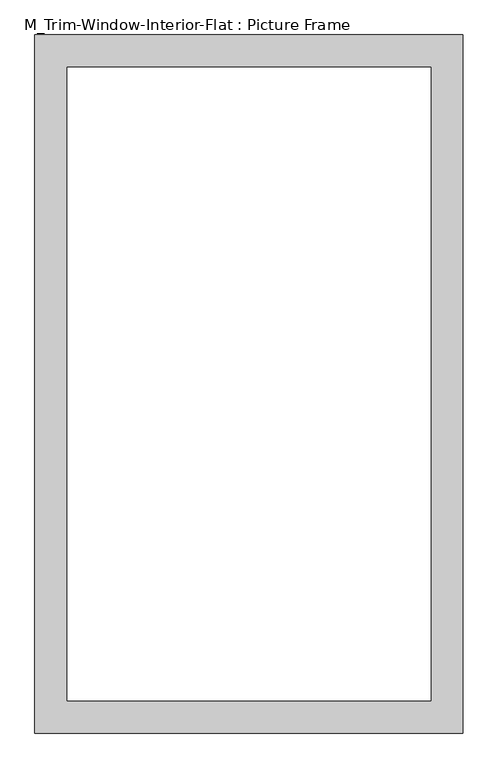
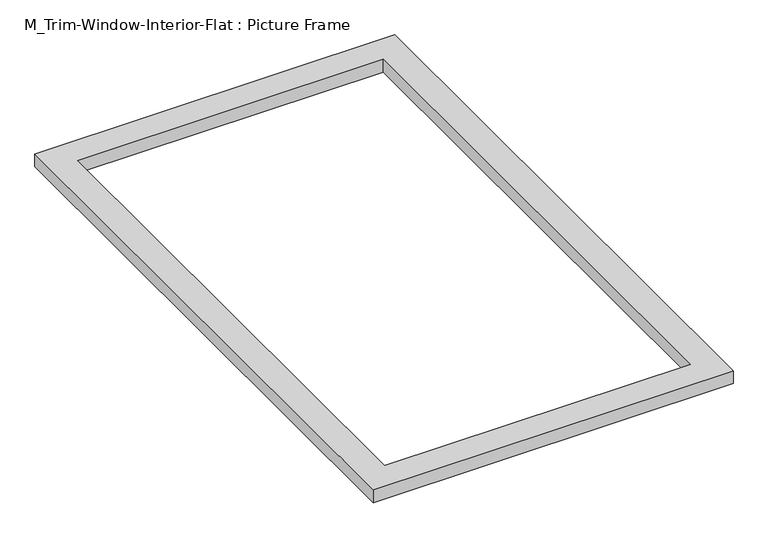
"""IFC4 building model written with IfcOpenShell, lengths in millimetres: proxy geometry, M_Trim-Window-Interior-Flat : Picture Frame."""

from ifc_helpers import new_model, si_unit, origin, origin_with_axes, place, context, project, spatial, polyline, outline, extrude, source, transform, mapped, element, save


def m_trim_window_interior_flat_picture_frame_c294611c(model_context):
    return source(origin(), model_context, "Body", "SweptSolid", [
        extrude(outline(polyline([(397.3, 47.3), (397.3, -1247.3), (-397.3, -1247.3), (-397.3, 47.3), (397.3, 47.3)]), holes=[polyline([(337.3, -12.7), (-337.3, -12.7), (-337.3, -1187.3), (337.3, -1187.3), (337.3, -12.7)])]), origin_with_axes(), (0.0, 0.0, 1.0), 30.0),
    ])


if __name__ == "__main__":
    model = new_model("IFC4")
    model_context = context("Model", 3, world=origin())
    ifc_project = project(units=[si_unit("LENGTHUNIT", "METRE", prefix="MILLI")], contexts=[model_context])
    site = spatial("IfcSite", under=ifc_project)
    building = spatial("IfcBuilding", under=site)
    placement = place(None, origin())
    m_trim_window_interior_flat_picture_frame_shape = m_trim_window_interior_flat_picture_frame_c294611c(model_context)
    element("IfcBuildingElementProxy", 1, Name="M_Trim-Window-Interior-Flat : Picture Frame", ObjectType="M_Trim-Window-Interior-Flat : Picture Frame", at=placement, inside=building, context=model_context, shape_type="MappedRepresentation", body=[
        mapped(m_trim_window_interior_flat_picture_frame_shape, transform((0.0, 0.0, 0.0), x_axis=(1.0, 0.0, 0.0), y_axis=(0.0, 1.0, 0.0), z_axis=(0.0, 0.0, 1.0))),
    ])
    save(model, "model.ifc")

# Revit data of these elements
# Type "M_Trim-Window-Interior-Flat : Picture Frame"
#   Trim Thickness_Picture Frame = 0.03 m
#   Trim Width = 0.06 m
#   Trim Thickness_with Sill = 0.02 m
#   Sill Thickness = 0.03 m
#   Opening Width [instance default] = 0.6 m
#   Opening Height [instance default] = 0.9 m
#   Default Elevation = 1.2 m
#   Sill = no
#   Picture Frame = yes
#   Trim Material [instance default] = none
# Element 1 (IfcBuildingElementProxy, "M_Trim-Window-Interior-Flat : Picture Frame")
#   Opening Width = 0.7 m
#   Opening Height = 1.2 m
#   Trim Material = Wood - Stained
#   Materials on its faces: "Wood - Stained"
# Materials
#   "Wood - Stained": class "Wood", colour RGB 224 178 126, transparency 0, Cost = 0
